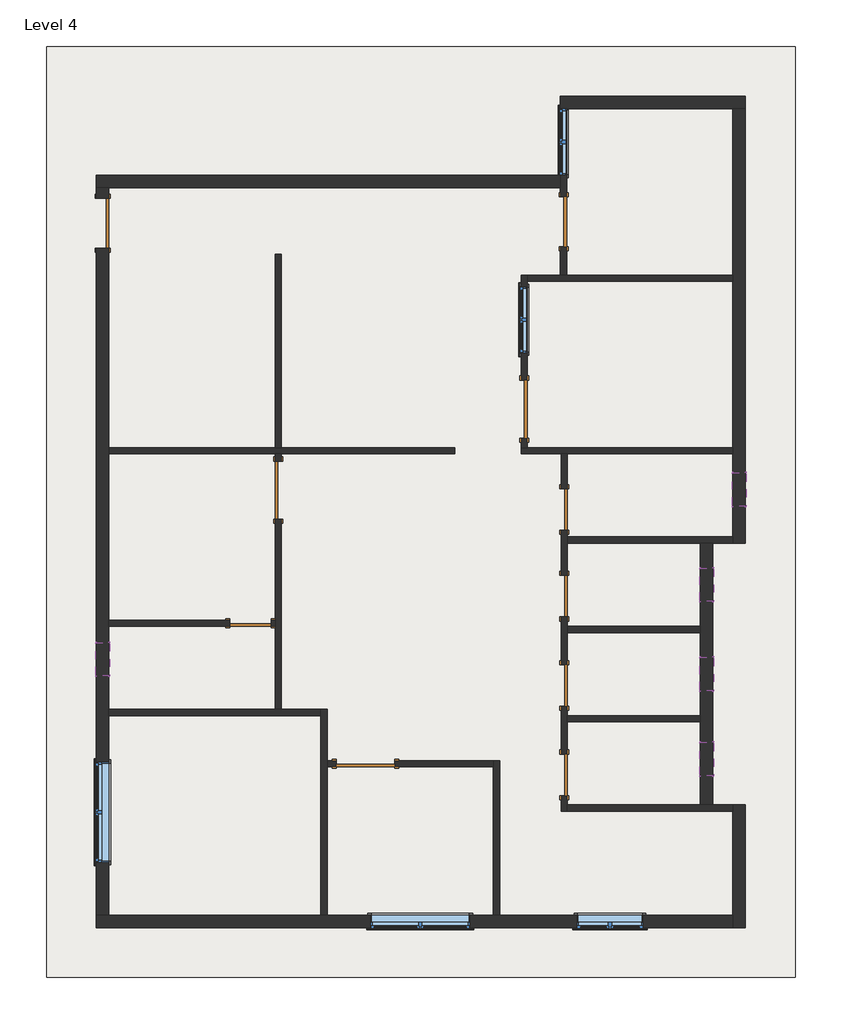
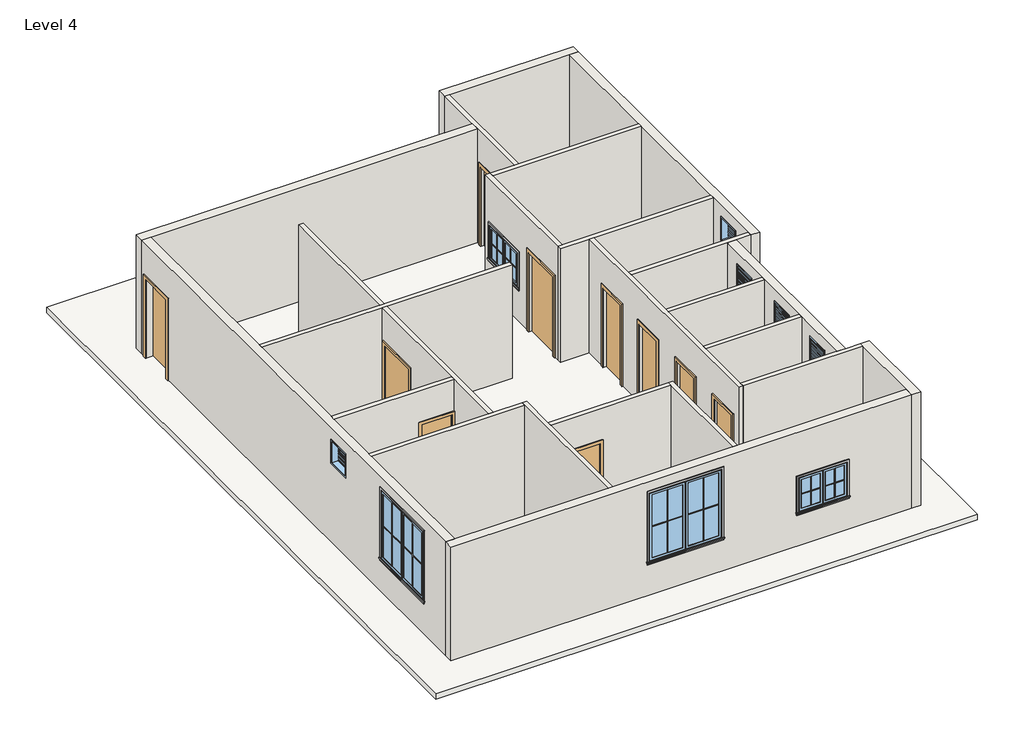
# One storey, incomplete: 23 walls, 20 proxies, 10 doors, 10 windows, 1 roof.
"""IFC4 building model written with IfcOpenShell, lengths in millimetres."""

from ifc_helpers import new_model, si_unit, frame, origin, place, context, project, spatial, polyline, outline, extrude, faceted_brep, transform, mapped, element, save
from components import muntin_pattern_2x2_muntin_pattern_2x2_0a037076, muntin_pattern_2x2_muntin_pattern_2x2_e6f69628, muntin_pattern_2x2_muntin_pattern_2x2_2357e71d, muntin_pattern_2x2_muntin_pattern_2x2_302d8f29, trim_window_exterior_flat_with_sill_b601e94a, trim_window_exterior_flat_with_sill_c4e67c73, trim_window_interior_flat_picture_frame_bfefb25c, trim_window_interior_flat_picture_frame_cf1733af, door_78caadf7, door_214872d5, single_flush_door_3_305aa2a5, single_flush_door_3_a90ba1ad, door_4c162e62, window_casement_double_win_4_c19c33cb, window_casement_double_win_4_2967420f, window_casement_double_win_6_ce442eab, window_f2d8fef0

model = new_model("IFC4")

# Units and contexts
model_context = context("Model", 3, world=origin())
ifc_project = project(units=[si_unit("LENGTHUNIT", "METRE", prefix="MILLI")], contexts=[model_context])

# Site, building, storey
site = spatial("IfcSite", under=ifc_project)
building = spatial("IfcBuilding", under=site)
storey = spatial("IfcBuildingStorey", under=building, Name="Level 4", Elevation=9448.8)

# Proxies
placement = place(None, origin())
muntin_pattern_2x2_muntin_pattern_2x2_shape = muntin_pattern_2x2_muntin_pattern_2x2_0a037076(model_context)
element("IfcBuildingElementProxy", 1, Name="Muntin Pattern_2x2 : Muntin Pattern_2x2", ObjectType="Muntin Pattern_2x2 : Muntin Pattern_2x2", at=placement, inside=storey, context=model_context, shape_type="MappedRepresentation", body=[
    mapped(muntin_pattern_2x2_muntin_pattern_2x2_shape, transform((-7058.058853, -4848.517381, 10433.05), x_axis=(0.0, 1.0, 0.0), y_axis=(-1.0, 0.0, 0.0), z_axis=(0.0, 0.0, 1.0))),
])
element("IfcBuildingElementProxy", 2, Name="Muntin Pattern_2x2 : Muntin Pattern_2x2", ObjectType="Muntin Pattern_2x2 : Muntin Pattern_2x2", at=placement, inside=storey, context=model_context, shape_type="MappedRepresentation", body=[
    mapped(muntin_pattern_2x2_muntin_pattern_2x2_shape, transform((-674.721353, -6497.929881, 10433.05), x_axis=(-1.0, 0.0, 0.0), y_axis=(0.0, -1.0, 0.0), z_axis=(0.0, 0.0, 1.0))),
])
muntin_pattern_2x2_muntin_pattern_2x2_2_shape = muntin_pattern_2x2_muntin_pattern_2x2_e6f69628(model_context)
element("IfcBuildingElementProxy", 3, Name="Muntin Pattern_2x2 : Muntin Pattern_2x2", ObjectType="Muntin Pattern_2x2 : Muntin Pattern_2x2", at=placement, inside=storey, context=model_context, shape_type="MappedRepresentation", body=[
    mapped(muntin_pattern_2x2_muntin_pattern_2x2_2_shape, transform((-7058.058853, -3937.292381, 10433.05), x_axis=(0.0, -1.0, 0.0), y_axis=(1.0, 0.0, 0.0), z_axis=(0.0, 0.0, 1.0))),
])
element("IfcBuildingElementProxy", 4, Name="Muntin Pattern_2x2 : Muntin Pattern_2x2", ObjectType="Muntin Pattern_2x2 : Muntin Pattern_2x2", at=placement, inside=storey, context=model_context, shape_type="MappedRepresentation", body=[
    mapped(muntin_pattern_2x2_muntin_pattern_2x2_2_shape, transform((-1585.946353, -6497.929881, 10433.05), x_axis=(1.0, 0.0, 0.0), y_axis=(0.0, 1.0, 0.0), z_axis=(0.0, 0.0, 1.0))),
])
muntin_pattern_2x2_muntin_pattern_2x2_3_shape = muntin_pattern_2x2_muntin_pattern_2x2_2357e71d(model_context)
element("IfcBuildingElementProxy", 5, Name="Muntin Pattern_2x2 : Muntin Pattern_2x2", ObjectType="Muntin Pattern_2x2 : Muntin Pattern_2x2", at=placement, inside=storey, context=model_context, shape_type="MappedRepresentation", body=[
    mapped(muntin_pattern_2x2_muntin_pattern_2x2_3_shape, transform((2652.678647, -6497.929881, 10433.05), x_axis=(-1.0, 0.0, 0.0), y_axis=(0.0, -1.0, 0.0), z_axis=(0.0, 0.0, 1.0))),
])
element("IfcBuildingElementProxy", 6, Name="Muntin Pattern_2x2 : Muntin Pattern_2x2", ObjectType="Muntin Pattern_2x2 : Muntin Pattern_2x2", at=placement, inside=storey, context=model_context, shape_type="MappedRepresentation", body=[
    mapped(muntin_pattern_2x2_muntin_pattern_2x2_3_shape, transform((727.041147, 4333.582619, 10433.05), x_axis=(0.0, 1.0, 0.0), y_axis=(-1.0, 0.0, 0.0), z_axis=(0.0, 0.0, 1.0))),
])
element("IfcBuildingElementProxy", 7, Name="Muntin Pattern_2x2 : Muntin Pattern_2x2", ObjectType="Muntin Pattern_2x2 : Muntin Pattern_2x2", at=placement, inside=storey, context=model_context, shape_type="MappedRepresentation", body=[
    mapped(muntin_pattern_2x2_muntin_pattern_2x2_3_shape, transform((1450.941147, 7591.132619, 10433.05), x_axis=(0.0, 1.0, 0.0), y_axis=(-1.0, 0.0, 0.0), z_axis=(0.0, 0.0, 1.0))),
])
muntin_pattern_2x2_muntin_pattern_2x2_4_shape = muntin_pattern_2x2_muntin_pattern_2x2_302d8f29(model_context)
element("IfcBuildingElementProxy", 8, Name="Muntin Pattern_2x2 : Muntin Pattern_2x2", ObjectType="Muntin Pattern_2x2 : Muntin Pattern_2x2", at=placement, inside=storey, context=model_context, shape_type="MappedRepresentation", body=[
    mapped(muntin_pattern_2x2_muntin_pattern_2x2_4_shape, transform((2046.253647, -6497.929881, 10433.05), x_axis=(1.0, 0.0, 0.0), y_axis=(0.0, 1.0, 0.0), z_axis=(0.0, 0.0, 1.0))),
])
element("IfcBuildingElementProxy", 9, Name="Muntin Pattern_2x2 : Muntin Pattern_2x2", ObjectType="Muntin Pattern_2x2 : Muntin Pattern_2x2", at=placement, inside=storey, context=model_context, shape_type="MappedRepresentation", body=[
    mapped(muntin_pattern_2x2_muntin_pattern_2x2_4_shape, transform((727.041147, 4940.007619, 10433.05), x_axis=(0.0, -1.0, 0.0), y_axis=(1.0, 0.0, 0.0), z_axis=(0.0, 0.0, 1.0))),
])
element("IfcBuildingElementProxy", 10, Name="Muntin Pattern_2x2 : Muntin Pattern_2x2", ObjectType="Muntin Pattern_2x2 : Muntin Pattern_2x2", at=placement, inside=storey, context=model_context, shape_type="MappedRepresentation", body=[
    mapped(muntin_pattern_2x2_muntin_pattern_2x2_4_shape, transform((1450.941147, 8197.557619, 10433.05), x_axis=(0.0, -1.0, 0.0), y_axis=(1.0, 0.0, 0.0), z_axis=(0.0, 0.0, 1.0))),
])
trim_window_exterior_flat_with_sill_shape = trim_window_exterior_flat_with_sill_b601e94a(model_context)
element("IfcBuildingElementProxy", 11, Name="Trim-Window-Exterior-Flat : with Sill", ObjectType="Trim-Window-Exterior-Flat : with Sill", at=placement, inside=storey, context=model_context, shape_type="MappedRepresentation", body=[
    mapped(trim_window_exterior_flat_with_sill_shape, transform((-7067.583853, -4392.904881, 12192.0), x_axis=(0.0, -1.0, 0.0), y_axis=(0.0, 0.0, 1.0), z_axis=(-1.0, 0.0, 0.0))),
])
element("IfcBuildingElementProxy", 12, Name="Trim-Window-Exterior-Flat : with Sill", ObjectType="Trim-Window-Exterior-Flat : with Sill", at=placement, inside=storey, context=model_context, shape_type="MappedRepresentation", body=[
    mapped(trim_window_exterior_flat_with_sill_shape, transform((-1130.333853, -6507.454881, 12192.0), x_axis=(1.0, 0.0, 0.0), y_axis=(0.0, 0.0, 1.0), z_axis=(0.0, -1.0, 0.0))),
])
trim_window_exterior_flat_with_sill_2_shape = trim_window_exterior_flat_with_sill_c4e67c73(model_context)
element("IfcBuildingElementProxy", 13, Name="Trim-Window-Exterior-Flat : with Sill", ObjectType="Trim-Window-Exterior-Flat : with Sill", at=placement, inside=storey, context=model_context, shape_type="MappedRepresentation", body=[
    mapped(trim_window_exterior_flat_with_sill_2_shape, transform((2349.466147, -6507.454881, 11277.6), x_axis=(1.0, 0.0, 0.0), y_axis=(0.0, 0.0, 1.0), z_axis=(0.0, -1.0, 0.0))),
])
element("IfcBuildingElementProxy", 14, Name="Trim-Window-Exterior-Flat : with Sill", ObjectType="Trim-Window-Exterior-Flat : with Sill", at=placement, inside=storey, context=model_context, shape_type="MappedRepresentation", body=[
    mapped(trim_window_exterior_flat_with_sill_2_shape, transform((717.516147, 4636.795119, 11277.6), x_axis=(0.0, -1.0, 0.0), y_axis=(0.0, 0.0, 1.0), z_axis=(-1.0, 0.0, 0.0))),
])
element("IfcBuildingElementProxy", 15, Name="Trim-Window-Exterior-Flat : with Sill", ObjectType="Trim-Window-Exterior-Flat : with Sill", at=placement, inside=storey, context=model_context, shape_type="MappedRepresentation", body=[
    mapped(trim_window_exterior_flat_with_sill_2_shape, transform((1441.416147, 7894.345119, 11277.6), x_axis=(0.0, -1.0, 0.0), y_axis=(0.0, 0.0, 1.0), z_axis=(-1.0, 0.0, 0.0))),
])
trim_window_interior_flat_picture_frame_shape = trim_window_interior_flat_picture_frame_bfefb25c(model_context)
element("IfcBuildingElementProxy", 16, Name="Trim-Window-Interior-Flat : Picture Frame", ObjectType="Trim-Window-Interior-Flat : Picture Frame", at=placement, inside=storey, context=model_context, shape_type="MappedRepresentation", body=[
    mapped(trim_window_interior_flat_picture_frame_shape, transform((-6838.983853, -4392.904881, 12192.0), x_axis=(0.0, 1.0, 0.0), y_axis=(0.0, 0.0, 1.0), z_axis=(1.0, 0.0, 0.0))),
])
element("IfcBuildingElementProxy", 17, Name="Trim-Window-Interior-Flat : Picture Frame", ObjectType="Trim-Window-Interior-Flat : Picture Frame", at=placement, inside=storey, context=model_context, shape_type="MappedRepresentation", body=[
    mapped(trim_window_interior_flat_picture_frame_shape, transform((-1130.333853, -6278.854881, 12192.0), x_axis=(-1.0, 0.0, 0.0), y_axis=(0.0, 0.0, 1.0), z_axis=(0.0, 1.0, 0.0))),
])
trim_window_interior_flat_picture_frame_2_shape = trim_window_interior_flat_picture_frame_cf1733af(model_context)
element("IfcBuildingElementProxy", 18, Name="Trim-Window-Interior-Flat : Picture Frame", ObjectType="Trim-Window-Interior-Flat : Picture Frame", at=placement, inside=storey, context=model_context, shape_type="MappedRepresentation", body=[
    mapped(trim_window_interior_flat_picture_frame_2_shape, transform((2349.466147, -6278.854881, 11277.6), x_axis=(-1.0, 0.0, 0.0), y_axis=(0.0, 0.0, 1.0), z_axis=(0.0, 1.0, 0.0))),
])
element("IfcBuildingElementProxy", 19, Name="Trim-Window-Interior-Flat : Picture Frame", ObjectType="Trim-Window-Interior-Flat : Picture Frame", at=placement, inside=storey, context=model_context, shape_type="MappedRepresentation", body=[
    mapped(trim_window_interior_flat_picture_frame_2_shape, transform((831.816147, 4636.795119, 11277.6), x_axis=(0.0, 1.0, 0.0), y_axis=(0.0, 0.0, 1.0), z_axis=(1.0, 0.0, 0.0))),
])
element("IfcBuildingElementProxy", 20, Name="Trim-Window-Interior-Flat : Picture Frame", ObjectType="Trim-Window-Interior-Flat : Picture Frame", at=placement, inside=storey, context=model_context, shape_type="MappedRepresentation", body=[
    mapped(trim_window_interior_flat_picture_frame_2_shape, transform((1555.716147, 7894.345119, 11277.6), x_axis=(0.0, 1.0, 0.0), y_axis=(0.0, 0.0, 1.0), z_axis=(1.0, 0.0, 0.0))),
])

# Doors
door_shape = door_78caadf7(model_context)
element("IfcDoor", 21, ObjectType="Single-Flush : 2'6\"", at=placement, inside=storey, context=model_context, shape_type="MappedRepresentation", body=[
    mapped(door_shape, transform((-4241.833853, -925.804881, 9448.8), x_axis=(1.0, 0.0, 0.0), y_axis=(0.0, 1.0, 0.0), z_axis=(0.0, 0.0, 1.0))),
])
door_2_shape = door_214872d5(model_context)
element("IfcDoor", 22, ObjectType="Single-Flush : 2'6\"", at=placement, inside=storey, context=model_context, shape_type="MappedRepresentation", body=[
    mapped(door_2_shape, transform((1511.266147, 1156.995119, 9448.8), x_axis=(0.0, -1.0, 0.0), y_axis=(1.0, 0.0, 0.0), z_axis=(0.0, 0.0, 1.0))),
])
element("IfcDoor", 23, ObjectType="Single-Flush : 2'6\"", at=placement, inside=storey, context=model_context, shape_type="MappedRepresentation", body=[
    mapped(door_2_shape, transform((1511.266147, -430.504881, 9448.8), x_axis=(0.0, -1.0, 0.0), y_axis=(1.0, 0.0, 0.0), z_axis=(0.0, 0.0, 1.0))),
])
element("IfcDoor", 24, ObjectType="Single-Flush : 2'6\"", at=placement, inside=storey, context=model_context, shape_type="MappedRepresentation", body=[
    mapped(door_2_shape, transform((1511.266147, -2068.804881, 9448.8), x_axis=(0.0, -1.0, 0.0), y_axis=(1.0, 0.0, 0.0), z_axis=(0.0, 0.0, 1.0))),
])
element("IfcDoor", 25, ObjectType="Single-Flush : 2'6\"", at=placement, inside=storey, context=model_context, shape_type="MappedRepresentation", body=[
    mapped(door_2_shape, transform((1511.266147, -3707.104881, 9448.8), x_axis=(0.0, -1.0, 0.0), y_axis=(1.0, 0.0, 0.0), z_axis=(0.0, 0.0, 1.0))),
])
single_flush_door_3_shape = single_flush_door_3_305aa2a5(model_context)
element("IfcDoor", 26, ObjectType="Single-Flush : DOOR 3'", at=placement, inside=storey, context=model_context, shape_type="MappedRepresentation", body=[
    mapped(single_flush_door_3_shape, transform((1498.566147, 6433.845119, 9448.8), x_axis=(0.0, 1.0, 0.0), y_axis=(-1.0, 0.0, 0.0), z_axis=(0.0, 0.0, 1.0))),
])
single_flush_door_3_2_shape = single_flush_door_3_a90ba1ad(model_context)
element("IfcDoor", 27, ObjectType="Single-Flush : DOOR 3'", at=placement, inside=storey, context=model_context, shape_type="MappedRepresentation", body=[
    mapped(single_flush_door_3_2_shape, transform((-6953.283853, 6408.445119, 9448.8), x_axis=(0.0, 1.0, 0.0), y_axis=(-1.0, 0.0, 0.0), z_axis=(0.0, 0.0, 1.0))),
])
door_3_shape = door_4c162e62(model_context)
element("IfcDoor", 28, ObjectType="Single-Flush : DOOR 3'6\"", at=placement, inside=storey, context=model_context, shape_type="MappedRepresentation", body=[
    mapped(door_3_shape, transform((-3733.833853, 1512.595119, 9448.8), x_axis=(0.0, 1.0, 0.0), y_axis=(-1.0, 0.0, 0.0), z_axis=(0.0, 0.0, 1.0))),
])
element("IfcDoor", 29, ObjectType="Single-Flush : DOOR 3'6\"", at=placement, inside=storey, context=model_context, shape_type="MappedRepresentation", body=[
    mapped(door_3_shape, transform((774.666147, 2998.495119, 9448.8), x_axis=(0.0, -1.0, 0.0), y_axis=(1.0, 0.0, 0.0), z_axis=(0.0, 0.0, 1.0))),
])
element("IfcDoor", 30, ObjectType="Single-Flush : DOOR 3'6\"", at=placement, inside=storey, context=model_context, shape_type="MappedRepresentation", body=[
    mapped(door_3_shape, transform((-2133.633853, -3503.904881, 9448.8), x_axis=(-1.0, 0.0, 0.0), y_axis=(0.0, -1.0, 0.0), z_axis=(0.0, 0.0, 1.0))),
])

# Roof
element("IfcRoof", 31, ObjectType="Generic - 12\"", at=placement, inside=storey, context=model_context, shape_type="SweptSolid", body=[
    extrude(outline(polyline([(-7981.983853, 9646.945119), (5746.716147, 9646.945119), (5746.716147, -7421.854881), (-7981.983853, -7421.854881), (-7981.983853, 9646.945119)])), frame((0.0, 0.0, 9296.4), z_axis=(0.0, 0.0, 1.0), x_axis=(1.0, 0.0, 0.0)), (0.0, 0.0, 1.0), 152.4),
])

# Walls
element("IfcWall", 32, ObjectType="WALL 4.5\"", at=placement, inside=storey, context=model_context, shape_type="Brep", body=[
    faceted_brep([(-6838.983853, 2179.345119, 9448.8), (-3790.983853, 2179.345119, 9448.8), (-3676.683853, 2179.345119, 9448.8), (-501.683853, 2179.345119, 9448.8), (-501.683853, 2179.345119, 12496.8), (-3676.683853, 2179.345119, 12496.8), (-3790.983853, 2179.345119, 12496.8), (-6838.983853, 2179.345119, 12496.8), (-6838.983853, 2293.645119, 9448.8), (-6838.983853, 2293.645119, 12496.8), (-3790.983853, 2293.645119, 12496.8), (-3676.683853, 2293.645119, 12496.8), (-501.683853, 2293.645119, 12496.8), (-501.683853, 2293.645119, 9448.8), (-3676.683853, 2293.645119, 9448.8), (-3790.983853, 2293.645119, 9448.8)], [[[0, 1, 2, 3, 4, 5, 6, 7]], [[8, 9, 10, 11, 12, 13, 14, 15]], [[3, 2, 1, 0, 8, 15, 14, 13]], [[4, 3, 13, 12]], [[0, 7, 9, 8]], [[7, 6, 5, 4, 12, 11, 10, 9]]]),
])
element("IfcWall", 33, ObjectType="WALL 4.5\"", at=placement, inside=storey, context=model_context, shape_type="Brep", body=[
    faceted_brep([(-2838.483853, -6278.854881, 9448.8), (-2838.483853, -3561.054881, 9448.8), (-2838.483853, -3446.754881, 9448.8), (-2838.483853, -2506.954881, 9448.8), (-2838.483853, -2506.954881, 12496.8), (-2838.483853, -3446.754881, 12496.8), (-2838.483853, -3561.054881, 12496.8), (-2838.483853, -6278.854881, 12496.8), (-2952.783853, -6278.854881, 9448.8), (-2952.783853, -6278.854881, 12496.8), (-2952.783853, -2621.254881, 12496.8), (-2952.783853, -2506.954881, 12496.8), (-2952.783853, -2506.954881, 9448.8), (-2952.783853, -2621.254881, 9448.8)], [[[0, 1, 2, 3, 4, 5, 6, 7]], [[8, 9, 10, 11, 12, 13]], [[3, 2, 1, 0, 8, 13, 12]], [[0, 7, 9, 8]], [[4, 3, 12, 11]], [[7, 6, 5, 4, 11, 10, 9]]]),
])
element("IfcWall", 34, ObjectType="WALL 4.5\"", at=placement, inside=storey, context=model_context, shape_type="Brep", body=[
    faceted_brep([(-2952.783853, -2506.954881, 9448.8), (-3676.683853, -2506.954881, 9448.8), (-3790.983853, -2506.954881, 9448.8), (-6838.983853, -2506.954881, 9448.8), (-6838.983853, -2506.954881, 12496.8), (-3790.983853, -2506.954881, 12496.8), (-3676.683853, -2506.954881, 12496.8), (-2952.783853, -2506.954881, 12496.8), (-2952.783853, -2621.254881, 9448.8), (-2952.783853, -2621.254881, 12496.8), (-6838.983853, -2621.254881, 12496.8), (-6838.983853, -2621.254881, 9448.8)], [[[0, 1, 2, 3, 4, 5, 6, 7]], [[8, 9, 10, 11]], [[3, 2, 1, 0, 8, 11]], [[0, 7, 9, 8]], [[4, 3, 11, 10]], [[7, 6, 5, 4, 10, 9]]]),
])
element("IfcWall", 35, ObjectType="WALL 4.5\"", at=placement, inside=storey, context=model_context, shape_type="SweptSolid", body=[
    extrude(outline(polyline([(11582.4, -3860.833853), (9448.8, -3860.833853), (9448.8, -3790.983853), (12496.8, -3790.983853), (12496.8, -6838.983853), (9448.8, -6838.983853), (9448.8, -4622.833853), (11582.4, -4622.833853), (11582.4, -3860.833853)])), frame((0.0, -982.954881, 0.0), z_axis=(0.0, 1.0, 0.0), x_axis=(0.0, 0.0, 1.0)), (0.0, 0.0, 1.0), 114.3),
])
element("IfcWall", 36, ObjectType="WALL 4.5\"", at=placement, inside=storey, context=model_context, shape_type="Brep", body=[
    faceted_brep([(-3676.683853, 5836.945119, 9448.8), (-3676.683853, 5836.945119, 12496.8), (-3676.683853, 2293.645119, 12496.8), (-3676.683853, 2293.645119, 9448.8), (-3790.983853, 5836.945119, 12496.8), (-3790.983853, 5836.945119, 9448.8), (-3790.983853, 2293.645119, 9448.8), (-3790.983853, 2293.645119, 12496.8)], [[[0, 1, 2, 3]], [[4, 5, 6, 7]], [[5, 0, 3, 6]], [[1, 0, 5, 4]], [[3, 2, 7, 6]], [[1, 4, 7, 2]]]),
    faceted_brep([(-3676.683853, -2506.954881, 12496.8), (-3676.683853, -2506.954881, 9448.8), (-3676.683853, 979.195119, 9448.8), (-3676.683853, 979.195119, 11582.4), (-3676.683853, 2045.995119, 11582.4), (-3676.683853, 2045.995119, 9448.8), (-3676.683853, 2179.345119, 9448.8), (-3676.683853, 2179.345119, 12496.8), (-3790.983853, -2506.954881, 9448.8), (-3790.983853, -2506.954881, 12496.8), (-3790.983853, -982.954881, 12496.8), (-3790.983853, -868.654881, 12496.8), (-3790.983853, 2179.345119, 12496.8), (-3790.983853, 2179.345119, 9448.8), (-3790.983853, 2045.995119, 9448.8), (-3790.983853, 2045.995119, 11582.4), (-3790.983853, 979.195119, 11582.4), (-3790.983853, 979.195119, 9448.8), (-3790.983853, -868.654881, 9448.8), (-3790.983853, -982.954881, 9448.8)], [[[0, 1, 2, 3, 4, 5, 6, 7]], [[8, 9, 10, 11, 12, 13, 14, 15, 16, 17, 18, 19]], [[1, 8, 19, 18, 17, 2]], [[5, 14, 13, 6]], [[1, 0, 9, 8]], [[7, 6, 13, 12]], [[15, 14, 5, 4]], [[16, 15, 4, 3]], [[17, 16, 3, 2]], [[9, 0, 7, 12, 11, 10]]]),
])
element("IfcWall", 37, ObjectType="WALL 4.5\"", at=placement, inside=storey, context=model_context, shape_type="Brep", body=[
    faceted_brep([(4603.716147, 2293.645119, 9448.8), (831.816147, 2293.645119, 9448.8), (717.516147, 2293.645119, 9448.8), (717.516147, 2293.645119, 12496.8), (831.816147, 2293.645119, 12496.8), (4603.716147, 2293.645119, 12496.8), (4603.716147, 2179.345119, 9448.8), (4603.716147, 2179.345119, 12496.8), (1568.416147, 2179.345119, 12496.8), (1454.116147, 2179.345119, 12496.8), (717.516147, 2179.345119, 12496.8), (717.516147, 2179.345119, 9448.8), (1454.116147, 2179.345119, 9448.8), (1568.416147, 2179.345119, 9448.8)], [[[0, 1, 2, 3, 4, 5]], [[6, 7, 8, 9, 10, 11, 12, 13]], [[2, 1, 0, 6, 13, 12, 11]], [[0, 5, 7, 6]], [[3, 2, 11, 10]], [[5, 4, 3, 10, 9, 8, 7]]]),
])
element("IfcWall", 38, ObjectType="WALL 4.5\"", at=placement, inside=storey, context=model_context, shape_type="Brep", body=[
    faceted_brep([(831.816147, 2293.645119, 9448.8), (831.816147, 2465.095119, 9448.8), (831.816147, 2465.095119, 11582.4), (831.816147, 3531.895119, 11582.4), (831.816147, 3531.895119, 9448.8), (831.816147, 5341.645119, 9448.8), (831.816147, 5455.945119, 9448.8), (831.816147, 5455.945119, 12496.8), (831.816147, 5341.645119, 12496.8), (831.816147, 2293.645119, 12496.8), (831.816147, 5246.395119, 11277.6), (831.816147, 5246.395119, 10363.2), (831.816147, 4027.195119, 10363.2), (831.816147, 4027.195119, 11277.6), (717.516147, 2465.095119, 11582.4), (717.516147, 2465.095119, 9448.8), (717.516147, 2293.645119, 9448.8), (717.516147, 2293.645119, 12496.8), (717.516147, 5455.945119, 12496.8), (717.516147, 5455.945119, 9448.8), (717.516147, 3531.895119, 9448.8), (717.516147, 3531.895119, 11582.4), (717.516147, 5246.395119, 11277.6), (717.516147, 4027.195119, 11277.6), (717.516147, 4027.195119, 10363.2), (717.516147, 5246.395119, 10363.2)], [[[0, 1, 2, 3, 4, 5, 6, 7, 8, 9], [10, 11, 12, 13]], [[14, 15, 16, 17, 18, 19, 20, 21], [22, 23, 24, 25]], [[20, 19, 6, 5, 4]], [[16, 15, 1, 0]], [[0, 9, 17, 16]], [[7, 6, 19, 18]], [[11, 10, 22, 25]], [[12, 11, 25, 24]], [[13, 12, 24, 23]], [[10, 13, 23, 22]], [[2, 1, 15, 14]], [[3, 2, 14, 21]], [[4, 3, 21, 20]], [[9, 8, 7, 18, 17]]]),
])
element("IfcWall", 39, ObjectType="WALL 4.5\"", at=placement, inside=storey, context=model_context, shape_type="Brep", body=[
    faceted_brep([(831.816147, 5341.645119, 9448.8), (4603.716147, 5341.645119, 9448.8), (4603.716147, 5341.645119, 12496.8), (831.816147, 5341.645119, 12496.8), (831.816147, 5455.945119, 9448.8), (831.816147, 5455.945119, 12496.8), (1441.416147, 5455.945119, 12496.8), (1555.716147, 5455.945119, 12496.8), (4603.716147, 5455.945119, 12496.8), (4603.716147, 5455.945119, 9448.8), (1555.716147, 5455.945119, 9448.8), (1441.416147, 5455.945119, 9448.8)], [[[0, 1, 2, 3]], [[4, 5, 6, 7, 8, 9, 10, 11]], [[1, 0, 4, 11, 10, 9]], [[0, 3, 5, 4]], [[2, 1, 9, 8]], [[3, 2, 8, 7, 6, 5]]]),
])
element("IfcWall", 40, ObjectType="WALL 4.5\"", at=placement, inside=storey, context=model_context, shape_type="Brep", body=[
    faceted_brep([(1555.716147, 6891.045119, 11582.4), (1555.716147, 6891.045119, 9448.8), (1555.716147, 8503.945119, 9448.8), (1555.716147, 8503.945119, 10363.2), (1555.716147, 7284.745119, 10363.2), (1555.716147, 7284.745119, 11277.6), (1555.716147, 8503.945119, 11277.6), (1555.716147, 8503.945119, 12496.8), (1555.716147, 5455.945119, 12496.8), (1555.716147, 5455.945119, 9448.8), (1555.716147, 5976.645119, 9448.8), (1555.716147, 5976.645119, 11582.4), (1441.416147, 8503.945119, 9448.8), (1441.416147, 7284.745119, 9448.8), (1441.416147, 7056.145119, 9448.8), (1441.416147, 6891.045119, 9448.8), (1441.416147, 6891.045119, 11582.4), (1441.416147, 5976.645119, 11582.4), (1441.416147, 5976.645119, 9448.8), (1441.416147, 5455.945119, 9448.8), (1441.416147, 5455.945119, 12496.8), (1441.416147, 7056.145119, 12496.8), (1441.416147, 7284.745119, 12496.8), (1441.416147, 8503.945119, 12496.8), (1441.416147, 8503.945119, 11277.6), (1441.416147, 7284.745119, 11277.6), (1441.416147, 7284.745119, 10363.2), (1441.416147, 8503.945119, 10363.2)], [[[0, 1, 2, 3, 4, 5, 6, 7, 8, 9, 10, 11]], [[12, 13, 14, 15, 16, 17, 18, 19, 20, 21, 22, 23, 24, 25, 26, 27]], [[10, 9, 19, 18]], [[2, 1, 15, 14, 13, 12]], [[24, 23, 7, 6]], [[12, 27, 3, 2]], [[9, 8, 20, 19]], [[4, 3, 27, 26]], [[5, 4, 26, 25]], [[6, 5, 25, 24]], [[16, 15, 1, 0]], [[17, 16, 0, 11]], [[18, 17, 11, 10]], [[8, 7, 23, 22, 21, 20]]]),
])
element("IfcWall", 41, ObjectType="WALL 4.5\"", at=placement, inside=storey, context=model_context, shape_type="Brep", body=[
    faceted_brep([(4603.716147, 655.345119, 9448.8), (1568.416147, 655.345119, 9448.8), (1568.416147, 655.345119, 12496.8), (4603.716147, 655.345119, 12496.8), (4603.716147, 541.045119, 9448.8), (4603.716147, 541.045119, 12496.8), (4235.416147, 541.045119, 12496.8), (4006.816147, 541.045119, 12496.8), (1568.416147, 541.045119, 12496.8), (1568.416147, 541.045119, 9448.8), (4006.816147, 541.045119, 9448.8), (4235.416147, 541.045119, 9448.8)], [[[0, 1, 2, 3]], [[4, 5, 6, 7, 8, 9, 10, 11]], [[1, 0, 4, 11, 10, 9]], [[0, 3, 5, 4]], [[2, 1, 9, 8]], [[3, 2, 8, 7, 6, 5]]]),
])
element("IfcWall", 42, ObjectType="WALL 4.5\"", at=placement, inside=storey, context=model_context, shape_type="Brep", body=[
    faceted_brep([(1454.116147, -4088.104881, 11582.4), (1454.116147, -4088.104881, 9448.8), (1454.116147, -4373.854881, 9448.8), (1454.116147, -4373.854881, 12496.8), (1454.116147, 2179.345119, 12496.8), (1454.116147, 2179.345119, 9448.8), (1454.116147, 1537.995119, 9448.8), (1454.116147, 1537.995119, 11582.4), (1454.116147, 775.995119, 11582.4), (1454.116147, 775.995119, 9448.8), (1454.116147, -49.504881, 9448.8), (1454.116147, -49.504881, 11582.4), (1454.116147, -811.504881, 11582.4), (1454.116147, -811.504881, 9448.8), (1454.116147, -1687.804881, 9448.8), (1454.116147, -1687.804881, 11582.4), (1454.116147, -2449.804881, 11582.4), (1454.116147, -2449.804881, 9448.8), (1454.116147, -3326.104881, 9448.8), (1454.116147, -3326.104881, 11582.4), (1568.416147, -4373.854881, 9448.8), (1568.416147, -4259.554881, 9448.8), (1568.416147, -4088.104881, 9448.8), (1568.416147, -4088.104881, 11582.4), (1568.416147, -3326.104881, 11582.4), (1568.416147, -3326.104881, 9448.8), (1568.416147, -2735.554881, 9448.8), (1568.416147, -2621.254881, 9448.8), (1568.416147, -2449.804881, 9448.8), (1568.416147, -2449.804881, 11582.4), (1568.416147, -1687.804881, 11582.4), (1568.416147, -1687.804881, 9448.8), (1568.416147, -1097.254881, 9448.8), (1568.416147, -982.954881, 9448.8), (1568.416147, -811.504881, 9448.8), (1568.416147, -811.504881, 11582.4), (1568.416147, -49.504881, 11582.4), (1568.416147, -49.504881, 9448.8), (1568.416147, 541.045119, 9448.8), (1568.416147, 655.345119, 9448.8), (1568.416147, 775.995119, 9448.8), (1568.416147, 775.995119, 11582.4), (1568.416147, 1537.995119, 11582.4), (1568.416147, 1537.995119, 9448.8), (1568.416147, 2179.345119, 9448.8), (1568.416147, 2179.345119, 12496.8), (1568.416147, 655.345119, 12496.8), (1568.416147, 541.045119, 12496.8), (1568.416147, -982.954881, 12496.8), (1568.416147, -1097.254881, 12496.8), (1568.416147, -2621.254881, 12496.8), (1568.416147, -2735.554881, 12496.8), (1568.416147, -4259.554881, 12496.8), (1568.416147, -4373.854881, 12496.8)], [[[0, 1, 2, 3, 4, 5, 6, 7, 8, 9, 10, 11, 12, 13, 14, 15, 16, 17, 18, 19]], [[20, 21, 22, 23, 24, 25, 26, 27, 28, 29, 30, 31, 32, 33, 34, 35, 36, 37, 38, 39, 40, 41, 42, 43, 44, 45, 46, 47, 48, 49, 50, 51, 52, 53]], [[6, 5, 44, 43]], [[10, 9, 40, 39, 38, 37]], [[14, 13, 34, 33, 32, 31]], [[18, 17, 28, 27, 26, 25]], [[2, 1, 22, 21, 20]], [[5, 4, 45, 44]], [[3, 2, 20, 53]], [[41, 40, 9, 8]], [[42, 41, 8, 7]], [[43, 42, 7, 6]], [[35, 34, 13, 12]], [[36, 35, 12, 11]], [[37, 36, 11, 10]], [[29, 28, 17, 16]], [[30, 29, 16, 15]], [[31, 30, 15, 14]], [[23, 22, 1, 0]], [[24, 23, 0, 19]], [[25, 24, 19, 18]], [[4, 3, 53, 52, 51, 50, 49, 48, 47, 46, 45]]]),
])
element("IfcWall", 43, ObjectType="WALL 4.5\"", at=placement, inside=storey, context=model_context, shape_type="Brep", body=[
    faceted_brep([(1568.416147, -4373.854881, 9448.8), (4603.716147, -4373.854881, 9448.8), (4603.716147, -4373.854881, 12496.8), (1568.416147, -4373.854881, 12496.8), (1568.416147, -4259.554881, 9448.8), (1568.416147, -4259.554881, 12496.8), (4006.816147, -4259.554881, 12496.8), (4235.416147, -4259.554881, 12496.8), (4603.716147, -4259.554881, 12496.8), (4603.716147, -4259.554881, 9448.8), (4235.416147, -4259.554881, 9448.8), (4006.816147, -4259.554881, 9448.8)], [[[0, 1, 2, 3]], [[4, 5, 6, 7, 8, 9, 10, 11]], [[1, 0, 4, 11, 10, 9]], [[0, 3, 5, 4]], [[2, 1, 9, 8]], [[3, 2, 8, 7, 6, 5]]]),
])
element("IfcWall", 44, ObjectType="WALL 4.5\"", at=placement, inside=storey, context=model_context, shape_type="SweptSolid", body=[
    extrude(outline(polyline([(4006.816147, -2735.554881), (1568.416147, -2735.554881), (1568.416147, -2621.254881), (4006.816147, -2621.254881), (4006.816147, -2735.554881)])), frame((0.0, 0.0, 9448.8), z_axis=(0.0, 0.0, 1.0), x_axis=(1.0, 0.0, 0.0)), (0.0, 0.0, 1.0), 3048.0),
])
element("IfcWall", 45, ObjectType="WALL 4.5\"", at=placement, inside=storey, context=model_context, shape_type="SweptSolid", body=[
    extrude(outline(polyline([(4006.816147, -1097.254881), (1568.416147, -1097.254881), (1568.416147, -982.954881), (4006.816147, -982.954881), (4006.816147, -1097.254881)])), frame((0.0, 0.0, 9448.8), z_axis=(0.0, 0.0, 1.0), x_axis=(1.0, 0.0, 0.0)), (0.0, 0.0, 1.0), 3048.0),
])
element("IfcWall", 46, ObjectType="WALL 4.5\"", at=placement, inside=storey, context=model_context, shape_type="Brep", body=[
    faceted_brep([(323.816147, -6278.854881, 9448.8), (323.816147, -3446.754881, 9448.8), (323.816147, -3446.754881, 12496.8), (323.816147, -6278.854881, 12496.8), (209.516147, -6278.854881, 9448.8), (209.516147, -6278.854881, 12496.8), (209.516147, -3561.054881, 12496.8), (209.516147, -3446.754881, 12496.8), (209.516147, -3446.754881, 9448.8), (209.516147, -3561.054881, 9448.8)], [[[0, 1, 2, 3]], [[4, 5, 6, 7, 8, 9]], [[1, 0, 4, 9, 8]], [[0, 3, 5, 4]], [[2, 1, 8, 7]], [[3, 2, 7, 6, 5]]]),
])
element("IfcWall", 47, ObjectType="WALL 4.5\"", at=placement, inside=storey, context=model_context, shape_type="SweptSolid", body=[
    extrude(outline(polyline([(9448.8, -2838.483853), (9448.8, -2667.033853), (11582.4, -2667.033853), (11582.4, -1600.233853), (9448.8, -1600.233853), (9448.8, 209.516147), (12496.8, 209.516147), (12496.8, -2838.483853), (9448.8, -2838.483853)])), frame((0.0, -3561.054881, 0.0), z_axis=(0.0, 1.0, 0.0), x_axis=(0.0, 0.0, 1.0)), (0.0, 0.0, 1.0), 114.3),
])
element("IfcWall", 48, ObjectType="WALL 9\"", at=placement, inside=storey, context=model_context, shape_type="Brep", body=[
    faceted_brep([(-7067.583853, 7056.145119, 9448.8), (-6838.983853, 7056.145119, 9448.8), (1441.416147, 7056.145119, 9448.8), (1441.416147, 7056.145119, 12496.8), (-6838.983853, 7056.145119, 12496.8), (-7067.583853, 7056.145119, 12496.8), (-7067.583853, 7284.745119, 9448.8), (-7067.583853, 7284.745119, 12496.8), (1441.416147, 7284.745119, 12496.8), (1441.416147, 7284.745119, 9448.8)], [[[0, 1, 2, 3, 4, 5]], [[6, 7, 8, 9]], [[2, 1, 0, 6, 9]], [[0, 5, 7, 6]], [[3, 2, 9, 8]], [[5, 4, 3, 8, 7]]]),
])
element("IfcWall", 49, ObjectType="WALL 9\"", at=placement, inside=storey, context=model_context, shape_type="Brep", body=[
    faceted_brep([(1441.416147, 8503.945119, 9448.8), (1555.716147, 8503.945119, 9448.8), (4603.716147, 8503.945119, 9448.8), (4832.316147, 8503.945119, 9448.8), (4832.316147, 8503.945119, 12496.8), (4603.716147, 8503.945119, 12496.8), (1555.716147, 8503.945119, 12496.8), (1441.416147, 8503.945119, 12496.8), (1441.416147, 8503.945119, 11277.6), (1441.416147, 8503.945119, 10363.2), (1441.416147, 8732.545119, 9448.8), (1441.416147, 8732.545119, 12496.8), (4832.316147, 8732.545119, 12496.8), (4832.316147, 8732.545119, 9448.8)], [[[0, 1, 2, 3, 4, 5, 6, 7, 8, 9]], [[10, 11, 12, 13]], [[3, 2, 1, 0, 10, 13]], [[4, 3, 13, 12]], [[0, 9, 8, 7, 11, 10]], [[7, 6, 5, 4, 12, 11]]]),
])
element("IfcWall", 50, ObjectType="WALL 9\"", at=placement, inside=storey, context=model_context, shape_type="Brep", body=[
    faceted_brep([(4603.716147, 8503.945119, 9448.8), (4603.716147, 5455.945119, 9448.8), (4603.716147, 5341.645119, 9448.8), (4603.716147, 2293.645119, 9448.8), (4603.716147, 2179.345119, 9448.8), (4603.716147, 655.345119, 9448.8), (4603.716147, 541.045119, 9448.8), (4603.716147, 541.045119, 12496.8), (4603.716147, 655.345119, 12496.8), (4603.716147, 2179.345119, 12496.8), (4603.716147, 2293.645119, 12496.8), (4603.716147, 5341.645119, 12496.8), (4603.716147, 5455.945119, 12496.8), (4603.716147, 8503.945119, 12496.8), (4603.716147, 1830.095119, 12192.0), (4603.716147, 1220.495119, 12192.0), (4603.716147, 1220.495119, 11582.4), (4603.716147, 1830.095119, 11582.4), (4832.316147, 8503.945119, 9448.8), (4832.316147, 8503.945119, 12496.8), (4832.316147, 541.045119, 12496.8), (4832.316147, 541.045119, 9448.8), (4832.316147, 1830.095119, 12192.0), (4832.316147, 1830.095119, 11582.4), (4832.316147, 1220.495119, 11582.4), (4832.316147, 1220.495119, 12192.0)], [[[0, 1, 2, 3, 4, 5, 6, 7, 8, 9, 10, 11, 12, 13], [14, 15, 16, 17]], [[18, 19, 20, 21], [22, 23, 24, 25]], [[6, 5, 4, 3, 2, 1, 0, 18, 21]], [[0, 13, 19, 18]], [[7, 6, 21, 20]], [[23, 22, 14, 17]], [[24, 23, 17, 16]], [[25, 24, 16, 15]], [[22, 25, 15, 14]], [[13, 12, 11, 10, 9, 8, 7, 20, 19]]]),
])
element("IfcWall", 51, ObjectType="WALL 9\"", at=placement, inside=storey, context=model_context, shape_type="Brep", body=[
    faceted_brep([(4006.816147, 541.045119, 9448.8), (4006.816147, -982.954881, 9448.8), (4006.816147, -1097.254881, 9448.8), (4006.816147, -2621.254881, 9448.8), (4006.816147, -2735.554881, 9448.8), (4006.816147, -4259.554881, 9448.8), (4006.816147, -4259.554881, 12496.8), (4006.816147, -2735.554881, 12496.8), (4006.816147, -2621.254881, 12496.8), (4006.816147, -1097.254881, 12496.8), (4006.816147, -982.954881, 12496.8), (4006.816147, 541.045119, 12496.8), (4006.816147, -525.754881, 12192.0), (4006.816147, -525.754881, 11582.4), (4006.816147, 83.845119, 11582.4), (4006.816147, 83.845119, 12192.0), (4006.816147, -2164.054881, 12192.0), (4006.816147, -2164.054881, 11582.4), (4006.816147, -1554.454881, 11582.4), (4006.816147, -1554.454881, 12192.0), (4006.816147, -3719.804881, 12192.0), (4006.816147, -3719.804881, 11582.4), (4006.816147, -3110.204881, 11582.4), (4006.816147, -3110.204881, 12192.0), (4235.416147, 541.045119, 9448.8), (4235.416147, 541.045119, 12496.8), (4235.416147, -4259.554881, 12496.8), (4235.416147, -4259.554881, 9448.8), (4235.416147, -525.754881, 12192.0), (4235.416147, 83.845119, 12192.0), (4235.416147, 83.845119, 11582.4), (4235.416147, -525.754881, 11582.4), (4235.416147, -2164.054881, 12192.0), (4235.416147, -1554.454881, 12192.0), (4235.416147, -1554.454881, 11582.4), (4235.416147, -2164.054881, 11582.4), (4235.416147, -3719.804881, 12192.0), (4235.416147, -3110.204881, 12192.0), (4235.416147, -3110.204881, 11582.4), (4235.416147, -3719.804881, 11582.4)], [[[0, 1, 2, 3, 4, 5, 6, 7, 8, 9, 10, 11], [12, 13, 14, 15], [16, 17, 18, 19], [20, 21, 22, 23]], [[24, 25, 26, 27], [28, 29, 30, 31], [32, 33, 34, 35], [36, 37, 38, 39]], [[5, 4, 3, 2, 1, 0, 24, 27]], [[0, 11, 25, 24]], [[6, 5, 27, 26]], [[13, 12, 28, 31]], [[14, 13, 31, 30]], [[15, 14, 30, 29]], [[12, 15, 29, 28]], [[17, 16, 32, 35]], [[18, 17, 35, 34]], [[19, 18, 34, 33]], [[16, 19, 33, 32]], [[21, 20, 36, 39]], [[22, 21, 39, 38]], [[23, 22, 38, 37]], [[20, 23, 37, 36]], [[11, 10, 9, 8, 7, 6, 26, 25]]]),
])
element("IfcWall", 52, ObjectType="WALL 9\"", at=placement, inside=storey, context=model_context, shape_type="Brep", body=[
    faceted_brep([(4603.716147, -4259.554881, 9448.8), (4603.716147, -4373.854881, 9448.8), (4603.716147, -6278.854881, 9448.8), (4603.716147, -6507.454881, 9448.8), (4603.716147, -6507.454881, 12496.8), (4603.716147, -6278.854881, 12496.8), (4603.716147, -4373.854881, 12496.8), (4603.716147, -4259.554881, 12496.8), (4832.316147, -4259.554881, 9448.8), (4832.316147, -4259.554881, 12496.8), (4832.316147, -6507.454881, 12496.8), (4832.316147, -6507.454881, 9448.8)], [[[0, 1, 2, 3, 4, 5, 6, 7]], [[8, 9, 10, 11]], [[3, 2, 1, 0, 8, 11]], [[4, 3, 11, 10]], [[0, 7, 9, 8]], [[7, 6, 5, 4, 10, 9]]]),
])
element("IfcWall", 53, ObjectType="WALL 9\"", at=placement, inside=storey, context=model_context, shape_type="Brep", body=[
    faceted_brep([(4603.716147, -6278.854881, 9448.8), (323.816147, -6278.854881, 9448.8), (209.516147, -6278.854881, 9448.8), (-2838.483853, -6278.854881, 9448.8), (-2952.783853, -6278.854881, 9448.8), (-6838.983853, -6278.854881, 9448.8), (-7067.583853, -6278.854881, 9448.8), (-7067.583853, -6278.854881, 12496.8), (-6838.983853, -6278.854881, 12496.8), (-2952.783853, -6278.854881, 12496.8), (-2838.483853, -6278.854881, 12496.8), (209.516147, -6278.854881, 12496.8), (323.816147, -6278.854881, 12496.8), (4603.716147, -6278.854881, 12496.8), (-2044.733853, -6278.854881, 12192.0), (-2044.733853, -6278.854881, 10363.2), (-215.933853, -6278.854881, 10363.2), (-215.933853, -6278.854881, 12192.0), (1739.866147, -6278.854881, 11277.6), (1739.866147, -6278.854881, 10363.2), (2959.066147, -6278.854881, 10363.2), (2959.066147, -6278.854881, 11277.6), (4603.716147, -6507.454881, 9448.8), (4603.716147, -6507.454881, 12496.8), (-7067.583853, -6507.454881, 12496.8), (-7067.583853, -6507.454881, 9448.8), (-2044.733853, -6507.454881, 12192.0), (-215.933853, -6507.454881, 12192.0), (-215.933853, -6507.454881, 10363.2), (-2044.733853, -6507.454881, 10363.2), (1739.866147, -6507.454881, 11277.6), (2959.066147, -6507.454881, 11277.6), (2959.066147, -6507.454881, 10363.2), (1739.866147, -6507.454881, 10363.2)], [[[0, 1, 2, 3, 4, 5, 6, 7, 8, 9, 10, 11, 12, 13], [14, 15, 16, 17], [18, 19, 20, 21]], [[22, 23, 24, 25], [26, 27, 28, 29], [30, 31, 32, 33]], [[6, 5, 4, 3, 2, 1, 0, 22, 25]], [[0, 13, 23, 22]], [[7, 6, 25, 24]], [[15, 14, 26, 29]], [[16, 15, 29, 28]], [[17, 16, 28, 27]], [[14, 17, 27, 26]], [[19, 18, 30, 33]], [[20, 19, 33, 32]], [[21, 20, 32, 31]], [[18, 21, 31, 30]], [[13, 12, 11, 10, 9, 8, 7, 24, 23]]]),
])
element("IfcWall", 54, ObjectType="WALL 9\"", at=placement, inside=storey, context=model_context, shape_type="Brep", body=[
    faceted_brep([(-6838.983853, 6865.645119, 11582.4), (-6838.983853, 6865.645119, 9448.8), (-6838.983853, 7056.145119, 9448.8), (-6838.983853, 7056.145119, 12496.8), (-6838.983853, 2293.645119, 12496.8), (-6838.983853, 2179.345119, 12496.8), (-6838.983853, -868.654881, 12496.8), (-6838.983853, -982.954881, 12496.8), (-6838.983853, -2506.954881, 12496.8), (-6838.983853, -2621.254881, 12496.8), (-6838.983853, -6278.854881, 12496.8), (-6838.983853, -6278.854881, 9448.8), (-6838.983853, -2621.254881, 9448.8), (-6838.983853, -2506.954881, 9448.8), (-6838.983853, -982.954881, 9448.8), (-6838.983853, -868.654881, 9448.8), (-6838.983853, 2179.345119, 9448.8), (-6838.983853, 2293.645119, 9448.8), (-6838.983853, 5951.245119, 9448.8), (-6838.983853, 5951.245119, 11582.4), (-6838.983853, -3478.504881, 12192.0), (-6838.983853, -3478.504881, 10363.2), (-6838.983853, -5307.304881, 10363.2), (-6838.983853, -5307.304881, 12192.0), (-6838.983853, -1281.404881, 12192.0), (-6838.983853, -1281.404881, 11582.4), (-6838.983853, -1891.004881, 11582.4), (-6838.983853, -1891.004881, 12192.0), (-7067.583853, 7056.145119, 9448.8), (-7067.583853, 6865.645119, 9448.8), (-7067.583853, 6865.645119, 11582.4), (-7067.583853, 5951.245119, 11582.4), (-7067.583853, 5951.245119, 9448.8), (-7067.583853, -6278.854881, 9448.8), (-7067.583853, -6278.854881, 12496.8), (-7067.583853, 7056.145119, 12496.8), (-7067.583853, -3478.504881, 12192.0), (-7067.583853, -5307.304881, 12192.0), (-7067.583853, -5307.304881, 10363.2), (-7067.583853, -3478.504881, 10363.2), (-7067.583853, -1281.404881, 12192.0), (-7067.583853, -1891.004881, 12192.0), (-7067.583853, -1891.004881, 11582.4), (-7067.583853, -1281.404881, 11582.4)], [[[0, 1, 2, 3, 4, 5, 6, 7, 8, 9, 10, 11, 12, 13, 14, 15, 16, 17, 18, 19], [20, 21, 22, 23], [24, 25, 26, 27]], [[28, 29, 30, 31, 32, 33, 34, 35], [36, 37, 38, 39], [40, 41, 42, 43]], [[2, 1, 29, 28]], [[18, 17, 16, 15, 14, 13, 12, 11, 33, 32]], [[11, 10, 34, 33]], [[3, 2, 28, 35]], [[21, 20, 36, 39]], [[22, 21, 39, 38]], [[23, 22, 38, 37]], [[20, 23, 37, 36]], [[25, 24, 40, 43]], [[26, 25, 43, 42]], [[27, 26, 42, 41]], [[24, 27, 41, 40]], [[30, 29, 1, 0]], [[31, 30, 0, 19]], [[32, 31, 19, 18]], [[10, 9, 8, 7, 6, 5, 4, 3, 35, 34]]]),
])

# Windows
window_casement_double_win_4_shape = window_casement_double_win_4_c19c33cb(model_context)
element("IfcWindow", 55, ObjectType="Window-Casement-Double : WIN 4'", at=placement, inside=storey, context=model_context, shape_type="MappedRepresentation", body=[
    mapped(window_casement_double_win_4_shape, transform((2349.466147, -6393.154881, 9448.8), x_axis=(-1.0, 0.0, 0.0), y_axis=(0.0, -1.0, 0.0), z_axis=(0.0, 0.0, 1.0))),
])
window_casement_double_win_4_2_shape = window_casement_double_win_4_2967420f(model_context)
element("IfcWindow", 56, ObjectType="Window-Casement-Double : WIN 4'", at=placement, inside=storey, context=model_context, shape_type="MappedRepresentation", body=[
    mapped(window_casement_double_win_4_2_shape, transform((774.666147, 4636.795119, 9448.8), x_axis=(0.0, 1.0, 0.0), y_axis=(-1.0, 0.0, 0.0), z_axis=(0.0, 0.0, 1.0))),
])
element("IfcWindow", 57, ObjectType="Window-Casement-Double : WIN 4'", at=placement, inside=storey, context=model_context, shape_type="MappedRepresentation", body=[
    mapped(window_casement_double_win_4_2_shape, transform((1498.566147, 7894.345119, 9448.8), x_axis=(0.0, 1.0, 0.0), y_axis=(-1.0, 0.0, 0.0), z_axis=(0.0, 0.0, 1.0))),
])
window_casement_double_win_6_shape = window_casement_double_win_6_ce442eab(model_context)
element("IfcWindow", 58, ObjectType="Window-Casement-Double : WIN 6'", at=placement, inside=storey, context=model_context, shape_type="MappedRepresentation", body=[
    mapped(window_casement_double_win_6_shape, transform((-6953.283853, -4392.904881, 9448.8), x_axis=(0.0, 1.0, 0.0), y_axis=(-1.0, 0.0, 0.0), z_axis=(0.0, 0.0, 1.0))),
])
element("IfcWindow", 59, ObjectType="Window-Casement-Double : WIN 6'", at=placement, inside=storey, context=model_context, shape_type="MappedRepresentation", body=[
    mapped(window_casement_double_win_6_shape, transform((-1130.333853, -6393.154881, 9448.8), x_axis=(-1.0, 0.0, 0.0), y_axis=(0.0, -1.0, 0.0), z_axis=(0.0, 0.0, 1.0))),
])
window_shape = window_f2d8fef0(model_context)
element("IfcWindow", 60, ObjectType="Window-Louvers : 24\" x 24\"", at=placement, inside=storey, context=model_context, shape_type="MappedRepresentation", body=[
    mapped(window_shape, transform((4724.366147, 1525.295119, 10668.0), x_axis=(0.0, -1.0, 0.0), y_axis=(1.0, 0.0, 0.0), z_axis=(0.0, 0.0, 1.0))),
])
element("IfcWindow", 61, ObjectType="Window-Louvers : 24\" x 24\"", at=placement, inside=storey, context=model_context, shape_type="MappedRepresentation", body=[
    mapped(window_shape, transform((4114.766147, -220.954881, 10668.0), x_axis=(0.0, 1.0, 0.0), y_axis=(-1.0, 0.0, 0.0), z_axis=(0.0, 0.0, 1.0))),
])
element("IfcWindow", 62, ObjectType="Window-Louvers : 24\" x 24\"", at=placement, inside=storey, context=model_context, shape_type="MappedRepresentation", body=[
    mapped(window_shape, transform((4114.766147, -1859.254881, 10668.0), x_axis=(0.0, 1.0, 0.0), y_axis=(-1.0, 0.0, 0.0), z_axis=(0.0, 0.0, 1.0))),
])
element("IfcWindow", 63, ObjectType="Window-Louvers : 24\" x 24\"", at=placement, inside=storey, context=model_context, shape_type="MappedRepresentation", body=[
    mapped(window_shape, transform((4114.766147, -3415.004881, 10668.0), x_axis=(0.0, 1.0, 0.0), y_axis=(-1.0, 0.0, 0.0), z_axis=(0.0, 0.0, 1.0))),
])
element("IfcWindow", 64, ObjectType="Window-Louvers : 24\" x 24\"", at=placement, inside=storey, context=model_context, shape_type="MappedRepresentation", body=[
    mapped(window_shape, transform((-6946.933853, -1586.204881, 10668.0), x_axis=(0.0, -1.0, 0.0), y_axis=(1.0, 0.0, 0.0), z_axis=(0.0, 0.0, 1.0))),
])

save(model, "model.ifc")

# Revit data of these elements
# Type "Muntin Pattern_2x2 : Muntin Pattern_2x2"
#   Width [instance default] = 4' - 0"
#   Thickness = 0' - 0 1/2"
#   Height [instance default] = 4' - 0"
#   Distance = 0' - 0 3/4"
#   Interior Material [instance default] = none
#   Exterior Material [instance default] = none
#   Default Elevation = 0
# Type "Trim-Window-Exterior-Flat : with Sill"
#   Trim Width = 0' - 2 1/4"
#   Trim Thickness_Picture Frame = 0' - 1 1/4"
#   Trim Thickness_with Sill = 0' - 0 3/4"
#   Sill Thickness = 0' - 1 1/4"
#   Opening Width [instance default] = 2' - 0"
#   Opening Height [instance default] = 3' - 0"
#   Default Elevation = 4' - 0"
#   Sill = yes
#   Picture Frame = no
#   Trim Material [instance default] = none
# Type "Trim-Window-Interior-Flat : Picture Frame"
#   Trim Thickness_Picture Frame = 0' - 1 1/4"
#   Trim Width = 0' - 2 1/4"
#   Trim Thickness_with Sill = 0' - 0 3/4"
#   Sill Thickness = 0' - 1 1/4"
#   Opening Width [instance default] = 2' - 0"
#   Opening Height [instance default] = 3' - 0"
#   Default Elevation = 4' - 0"
#   Sill = no
#   Picture Frame = yes
#   Trim Material [instance default] = none
# Type "Single-Flush : 2'6\""
#   Type Mark = "10"
#   Construction Type Id = "MDOOR"
#   Assembly Code = "C1020"
#   Analytic Construction = "Metal"
#   Thickness = 0' - 2"
#   Heat Transfer Coefficient (U) = 0.651978 BTU/(h·ft²·°F)
#   Height = 7' - 0"
#   Trim Projection Ext = 0' - 1"
#   Trim Projection Int = 0' - 1"
#   Trim Width = 0' - 3"
#   Width = 2' - 6"
#   Define Thermal Properties by = 1
#   Door Material = Door - Panel
#   Frame Material = Door - Frame
#   Visual Light Transmittance = 0
#   Solar Heat Gain Coefficient = 0
#   Function = (empty or 0)
#   Wall Closure = (empty or 0)
# Type "Single-Flush : DOOR 3'"
#   Type Mark = "8"
#   Construction Type Id = "MDOOR"
#   Assembly Code = "C1020"
#   Analytic Construction = "Metal"
#   Thickness = 0' - 2"
#   Heat Transfer Coefficient (U) = 0.651978 BTU/(h·ft²·°F)
#   Height = 7' - 0"
#   Trim Projection Ext = 0' - 1"
#   Trim Projection Int = 0' - 1"
#   Trim Width = 0' - 3"
#   Width = 3' - 0"
#   Define Thermal Properties by = 1
#   Door Material = Door - Panel
#   Frame Material = Door - Frame
#   Visual Light Transmittance = 0
#   Solar Heat Gain Coefficient = 0
#   Function = (empty or 0)
#   Wall Closure = (empty or 0)
# Type "Single-Flush : DOOR 3'6\""
#   Type Mark = "9"
#   Construction Type Id = "MDOOR"
#   Assembly Code = "C1020"
#   Analytic Construction = "Metal"
#   Thickness = 0' - 2"
#   Heat Transfer Coefficient (U) = 0.651978 BTU/(h·ft²·°F)
#   Height = 7' - 0"
#   Trim Projection Ext = 0' - 1"
#   Trim Projection Int = 0' - 1"
#   Trim Width = 0' - 3"
#   Width = 3' - 6"
#   Define Thermal Properties by = 1
#   Door Material = Door - Panel
#   Frame Material = Door - Frame
#   Visual Light Transmittance = 0
#   Solar Heat Gain Coefficient = 0
#   Function = (empty or 0)
#   Wall Closure = (empty or 0)
# Type "Generic - 12\""
#   Assembly Code = "B1020"
#   Layers, outside or top first: 0' - 6" no material (function 1)
# Type "WALL 4.5\""
#   Assembly Code = "B2010"
#   Layers, outside or top first: 0' - 4 1/2" no material (function 1)
# Type "WALL 9\""
#   Assembly Code = "B2010"
#   Layers, outside or top first: 0' - 9" no material (function 1)
# Type "Window-Casement-Double : WIN 4'"
#   Type Mark = "18"
#   Fire Rating = "0.5h"
#   Assembly Code = "B2020100"
#   Analytic Construction = "Double glazing - domestic"
#   Frame Extension [instance default] = 0' - 0 1/4"
#   Window Inset [instance default] = 0' - 0"
#   Wall Thickness [instance default] = 0' - 6"
#   Interior Wall Closure [instance default] = 0' - 2 1/4"
#   Half Width = 2' - 0"
#   Visual Light Transmittance = 0.81
#   Thermal Resistance (R) = 1.8146 (h·ft²·°F)/BTU
#   Solar Heat Gain Coefficient = 0.76
#   Rough Width = 4' - 0 1/2"
#   Rough Height = 3' - 0 1/2"
#   Height = 3' - 0"
#   Heat Transfer Coefficient (U) = 0.5511 BTU/(h·ft²·°F)
#   Exterior Wall Closure [instance default] = 0' - 1 1/4"
#   Extension Jamb [instance default] = 0' - 2 1/4"
#   Default Sill Height = 3' - 0"
#   Width = 4' - 0"
#   Muntin Visibility = yes
#   Interior Trim Visibility [instance default] = yes
#   Exterior Trim Visibility [instance default] = yes
#   Extension Jamb Visibility [instance default] = yes
#   Interior Trim Material = Wood - Stained
#   Muntin Pattern = Muntin Pattern_2x2 : Muntin Pattern_2x2
#   Interior Trim = Trim-Window-Interior-Flat : Picture Frame
#   Interior Frame Material = Wood - Stained
#   Glass Panel Material = Glass
#   Exterior Trim Material = Clad - White
#   Exterior Trim = Trim-Window-Exterior-Flat : with Sill
#   Exterior Frame Material = Clad - White
#   Wall Closure = (empty or 0)
# Type "Window-Casement-Double : WIN 6'"
#   Type Mark = "19"
#   Fire Rating = "0.5h"
#   Assembly Code = "B2020100"
#   Analytic Construction = "Double glazing - domestic"
#   Frame Extension [instance default] = 0' - 0 1/4"
#   Window Inset [instance default] = 0' - 0"
#   Wall Thickness [instance default] = 0' - 6"
#   Interior Wall Closure [instance default] = 0' - 2 1/4"
#   Half Width = 3' - 0"
#   Visual Light Transmittance = 0.81
#   Thermal Resistance (R) = 1.8146 (h·ft²·°F)/BTU
#   Solar Heat Gain Coefficient = 0.76
#   Rough Width = 6' - 0 1/2"
#   Rough Height = 6' - 0 1/2"
#   Height = 6' - 0"
#   Heat Transfer Coefficient (U) = 0.5511 BTU/(h·ft²·°F)
#   Exterior Wall Closure [instance default] = 0' - 1 1/4"
#   Extension Jamb [instance default] = 0' - 2 1/4"
#   Default Sill Height = 3' - 0"
#   Width = 6' - 0"
#   Muntin Visibility = yes
#   Interior Trim Visibility [instance default] = yes
#   Exterior Trim Visibility [instance default] = yes
#   Extension Jamb Visibility [instance default] = yes
#   Interior Trim Material = Wood - Stained
#   Muntin Pattern = Muntin Pattern_2x2 : Muntin Pattern_2x2
#   Interior Trim = Trim-Window-Interior-Flat : Picture Frame
#   Interior Frame Material = Wood - Stained
#   Glass Panel Material = Glass
#   Exterior Trim Material = Clad - White
#   Exterior Trim = Trim-Window-Exterior-Flat : with Sill
#   Exterior Frame Material = Clad - White
#   Wall Closure = (empty or 0)
# Type "Window-Louvers : 24\" x 24\""
#   Type Mark = "20"
#   Construction Type Id = "GSP4R"
#   Assembly Code = "B20"
#   Analytic Construction = "1/8 in Pilkington single glazing"
#   Visual Light Transmittance = 0.9
#   Thermal Resistance (R) = 1.53941 (h·ft²·°F)/BTU
#   Solar Heat Gain Coefficient = 0.78
#   Max Height = 1' - 11.74264"
#   Height = 2' - 0"
#   Heat Transfer Coefficient (U) = 0.6496 BTU/(h·ft²·°F)
#   Blade Width [instance default] = 1' - 10 1/2"
#   Blade Vertical Thickness = 0' - 0.35355"
#   Blade Thickness = 0' - 0 1/4"
#   Blade Spacing = 0' - 1 1/2"
#   Blade Height = 0' - 1.85355"
#   Blade Depth = 0' - 3"
#   Blade Angle = 45.00°
#   Default Sill Height = 3' - 0"
#   Trim Projection_Exterior = 0' - 0 1/2"
#   Trim Projection_Interior = 0' - 0 1/2"
#   Trim Width_Exterior = 0' - 1 1/2"
#   Trim Width_Interior = 0' - 1 1/2"
#   Width = 2' - 0"
#   Max Blade Count = 12
#   Define Thermal Properties by = 1
#   Blade Count = 12
#   Frame Material = Birch
#   Louver Material = Birch
#   Trim Exterior Material = Birch
#   Trim Interior Material = Birch
#   Wall Closure = (empty or 0)
# Elements 1, 2, 3, 4 (IfcBuildingElementProxy, "Muntin Pattern_2x2 : Muntin Pattern_2x2")
#   Width = 2' - 6 5/8"
#   Height = 5' - 6 1/2"
#   Interior Material = Wood - Stained
#   Exterior Material = Clad - White
#   Phase Created = New Construction
#   Materials on its faces: "Clad - White", "Wood - Stained"
# Elements 5, 6, 7, 8, 9, 10 (IfcBuildingElementProxy, "Muntin Pattern_2x2 : Muntin Pattern_2x2")
#   Width = 1' - 6 5/8"
#   Height = 2' - 6 1/2"
#   Interior Material = Wood - Stained
#   Exterior Material = Clad - White
#   Phase Created = New Construction
#   Materials on its faces: "Clad - White", "Wood - Stained"
# Elements 11, 12 (IfcBuildingElementProxy, "Trim-Window-Exterior-Flat : with Sill")
#   Opening Width = 6' - 0"
#   Opening Height = 6' - 0"
#   Trim Material = Clad - White
#   Phase Created = New Construction
#   Materials on its faces: "Clad - White"
# Elements 13, 14, 15 (IfcBuildingElementProxy, "Trim-Window-Exterior-Flat : with Sill")
#   Opening Width = 4' - 0"
#   Opening Height = 3' - 0"
#   Trim Material = Clad - White
#   Phase Created = New Construction
#   Materials on its faces: "Clad - White"
# Elements 16, 17 (IfcBuildingElementProxy, "Trim-Window-Interior-Flat : Picture Frame")
#   Opening Width = 6' - 0"
#   Opening Height = 6' - 0"
#   Trim Material = Wood - Stained
#   Phase Created = New Construction
#   Materials on its faces: "Wood - Stained"
# Elements 18, 19, 20 (IfcBuildingElementProxy, "Trim-Window-Interior-Flat : Picture Frame")
#   Opening Width = 4' - 0"
#   Opening Height = 3' - 0"
#   Trim Material = Wood - Stained
#   Phase Created = New Construction
#   Materials on its faces: "Wood - Stained"
# Elements 21, 22, 23, 24, 25 (IfcDoor, "Single-Flush : 2'6\"")
#   Phase Created = New Construction
#   Materials on its faces: "Door - Frame", "Door - Panel"
# Elements 26, 27 (IfcDoor, "Single-Flush : DOOR 3'")
#   Phase Created = New Construction
#   Materials on its faces: "Door - Frame", "Door - Panel"
# Elements 28, 29, 30 (IfcDoor, "Single-Flush : DOOR 3'6\"")
#   Phase Created = New Construction
#   Materials on its faces: "Door - Frame", "Door - Panel"
# Element 31 (IfcRoof, "Generic - 12\"")
#   built-in parameter 1001705 = 31 (stored number, unit not read)
#   built-in parameter 1001701 = -0.5 (stored number, unit not read)
#   built-in parameter 1001710 = 33615
#   Phase Created = New Construction
#   Materials on its faces: "Default Roof", "Cherry", "Wood Planks"
# Elements 32, 33, 34, 35, 36, 37, 38, 39, 42, 43, 44, 45, 46, 47 (IfcWall, "WALL 4.5\"")
#   Top Offset = 0' - 0"
#   Base Offset = 0' - 0"
#   Unconnected Height = 10' - 0"
#   wall height = 10' - 0"
#   Phase Created = New Construction
#   Base Constraint = Level 4
#   Materials on its faces: "Default Wall"
# Elements 40, 41 (IfcWall, "WALL 4.5\"")
#   Top Offset = 0' - 0"
#   Base Offset = 0' - 0"
#   Unconnected Height = 10' - 0"
#   wall height = 10' - 0"
#   Phase Created = New Construction
#   Base Constraint = Level 4
#   Materials on its faces: "Default Wall", "Wood - Stained"
# Elements 48, 49, 50, 51, 52, 53, 54 (IfcWall, "WALL 9\"")
#   Top Offset = 0' - 0"
